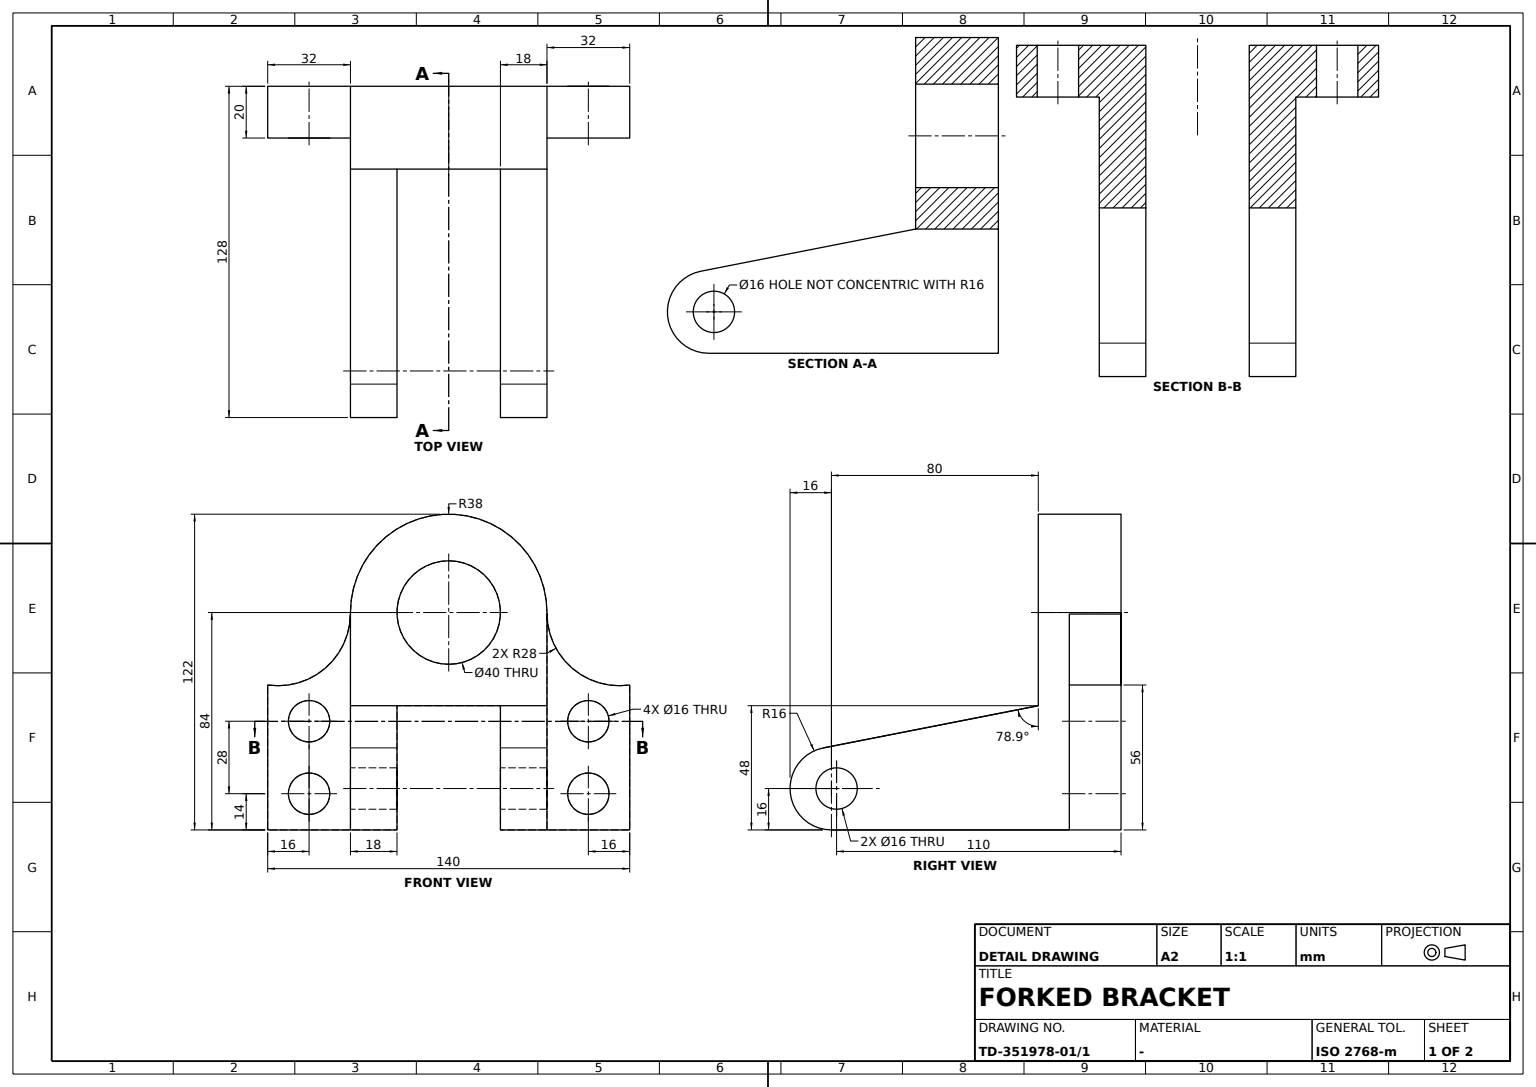
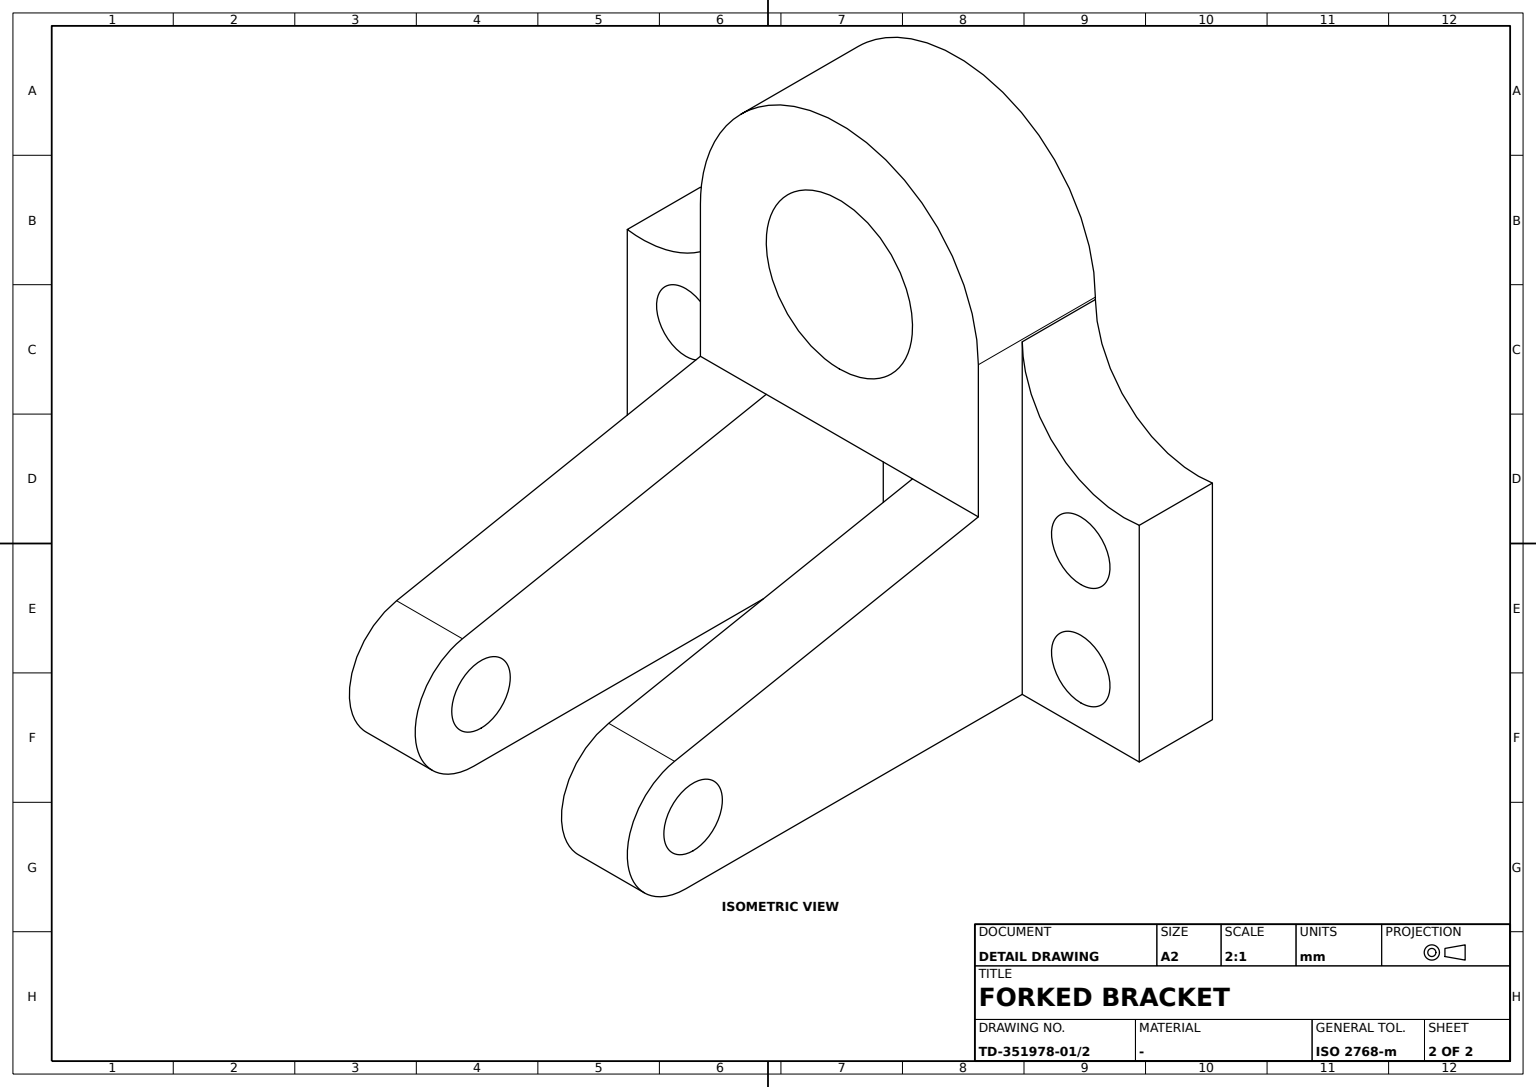
CATIA V5 part; units mm, degrees
sketch "Sketch1" plane through (0, 0, 0) normal (1, 0, 0) x (0, 1, 0)
  line L0 (0, 149.0848) -> (0, -86.9094) construction
  point P0 (0, 149.0848)
  point P1 (-20, 0)
  line L1 (-20, 0) -> (-38, 0)
  line L2 (-38, 0) -> (-38, 48)
  line L3 (38, 48) -> (38, 0)
  point P2 (38, 0)
  line L4 (38, 0) -> (20, 0)
  line L5 (20, 0) -> (20, 48)
  line L6 (-20, 48) -> (-20, 0)
  point P3 (0, 84)
  line L7 (-38, 48) -> (-20, 48)
  line L8 (20, 48) -> (38, 48)
  dimension "distance L6 L5" = 40
  dimension "distance L6 L0" = 20
  dimension "distance L2 L0" = 38
  dimension "length L6" = 48
  dimension "distance P3 L4" = 84
  dimension "length L3" = 48
  dimension "length L8" = 18
  constraint coincidence P0 y-axis
  constraint coincidence P1 x-axis
  constraint coincidence P2 x-axis
  constraint vertical L0 y-axis
  constraint vertical L2 y-axis
  constraint vertical L3 y-axis
  constraint vertical L5 y-axis
  constraint vertical L6 y-axis
  constraint horizontal L1 x-axis
  constraint horizontal L4 x-axis
  constraint horizontal L7 x-axis
  constraint horizontal L8 x-axis
extrude "Pad1" add sketch "Sketch1" along normal mid plane 32
sketch "Sketch2" plane through (16, 0, 0) normal (1, 0, 0) x (0, 1, 0)
  point P0 (-38, 48)
  line L0 (-38, 48) -> (-38, 84)
  line L1 (38, 84) -> (38, 48)
  point P1 (38, 48)
  line L2 (38, 48) -> (-38, 48)
  point P2 (-38, 48)
  point P3 (38, 48)
  arc A0 (-38, 84) -> (38, 84) centre (0, 84) cw
  dimension "length L1" = 36
  constraint vertical L0 y-axis
  constraint vertical L1 y-axis
  constraint horizontal L2 x-axis
  constraint coincidence P2 P0
  constraint coincidence P1 P3
  constraint tangency A0 L1
  constraint tangency A0 L0
extrude "Pad2" add sketch "Sketch2" against normal blind 32
sketch "Sketch3" plane through (16, 0, 0) normal (1, 0, 0) x (0, 1, 0)
  circle A0 centre (0, 84) radius 20
  point P0 (0, 84)
  arc A1 (38, 84) -> (-38, 84) centre (0, 84) ccw construction
  dimension "radius A0" = 20
  dimension "distance A0 A1" = 18
  constraint coincidence P0 y-axis
extrude "Pocket1" cut sketch "Sketch3" against normal blind 32
sketch "Sketch4" plane through (0, -38, 0) normal (0, -1, 0) x (1, 0, 0)
  point P0 (16, 0)
  line L0 (16, 0) -> (96, 0)
  line L1 (99.0803, 31.7007) -> (16, 48)
  point P1 (16, 48)
  line L2 (16, 48) -> (16, 0)
  line L3 (16, 48) -> (16, 0) construction
  arc A0 (99.0803, 31.7007) -> (96, 0) centre (96, 16) cw
  dimension "length L2" = 48
  dimension "length L0" = 80
  dimension "radius A0" = 16
  constraint coincidence P0 x-axis
  constraint coincidence P1 L3
  constraint horizontal L0 x-axis
  constraint vertical L2 y-axis
  constraint tangency A0 L0
  constraint tangency A0 L1
extrude "Pad3" add sketch "Sketch4" against normal blind 18
sketch "Sketch5" plane through (-16, 0, 0) normal (-1, 0, 0) x (0, -1, 0)
  point P0 (38, 0)
  line L0 (38, 0) -> (70, 0)
  line L1 (70, 0) -> (70, 56)
  arc A0 (70, 56) -> (38, 84) centre (65.9985, 83.7126) cw
  point P1 (38, 84)
  line L2 (38, 84) -> (38, 0)
  point P2 (38, 84)
  point P3 (38, 0)
  dimension "radius A0" = 28
  dimension "length L0" = 32
  dimension "length L1" = 56
  constraint coincidence P0 x-axis
  constraint coincidence P1 P2
  constraint coincidence P0 P3
  constraint horizontal L0 x-axis
  constraint vertical L1 y-axis
extrude "Pad4" add sketch "Sketch5" against normal blind 20
mirror "Mirror1" about plane through (0, 0, 0) normal (0, 1, 0) of "Pad3", "Pad4"
sketch "Sketch6" plane through (4, 0, 0) normal (1, 0, 0) x (0, 1, 0)
  circle A0 centre (-54, 42) radius 8
  point P0 (-54, 42)
  circle A1 centre (-54, 14) radius 8
  point P1 (-54, 14)
  point P2 (-70, 56)
  line L0 (-70, 0) -> (-70, 56) construction
  line L1 (-70, 0) -> (-70, 56) construction
  dimension "radius A0" = 8
  dimension "radius A1" = 8
  dimension "distance P0 P2 y axis" = 14
  dimension "distance P0 P1" = 28
  dimension "distance P1 L0" = 16
  dimension "distance P0 L1" = 16
extrude "Pocket2" cut sketch "Sketch6" against normal blind 20
mirror "Mirror2" about plane through (0, 0, 0) normal (0, 1, 0) of "Pocket2"
sketch "Sketch7" plane through (0, -38, 0) normal (0, -1, 0) x (1, 0, 0)
  circle A0 centre (94, 16) radius 8
  point P0 (94, 16)
  line L0 (-16, 0) -> (-16, 56) construction
  line L1 (-16, 0) -> (16, 0) construction
  dimension "radius A0" = 8
  dimension "distance P0 L0" = 110
  dimension "distance P0 L1" = 16
extrude "Pocket3" cut sketch "Sketch7" against normal blind 89
